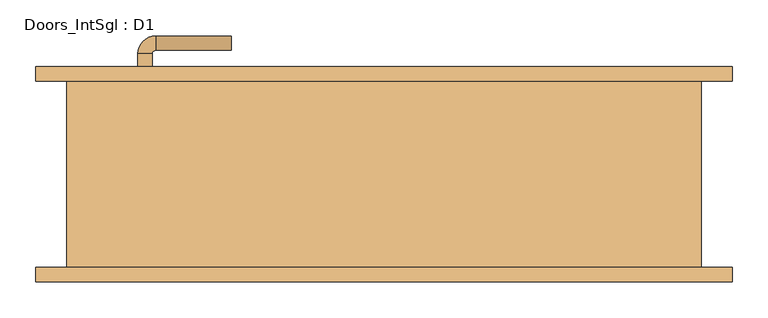
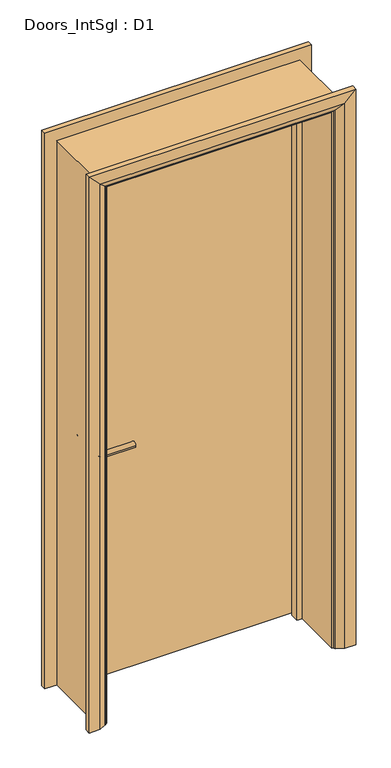
"""IFC4 building model written with IfcOpenShell, lengths in millimetres: door geometry, Doors_IntSgl : D1."""

from ifc_helpers import new_model, si_unit, point, frame, frame_2d, origin, place, context, project, spatial, polyline, circle_curve, ellipse_curve, trimmed, segment, composite_curve, outline, extrude, faceted_brep, source, transform, mapped, element, save
from ifc_brep_helpers import plane_surface, cylinder_surface, revolved_surface, advanced_brep


def doors_intsgl_d1_8eed65bb(model_context):
    return source(origin(), model_context, "Body", "SolidModel", [
        advanced_brep(
        [(-343.0, 84.0, 900.0), (-323.0, 84.0, 900.0), (-323.0, 54.0, 900.0), (-343.0, 54.0, 900.0), (-318.0, 49.0, 900.0), (-318.0, 29.0, 900.0), (-213.0, 29.0, 900.0), (-213.0, 49.0, 900.0)],
        [
            (0, 1, circle_curve(frame((-333.0, 84.0, 900.0), z_axis=(0.0, 1.0, 0.0), x_axis=(1.0, 0.0, 0.0)), 10.0)),
            (1, 0, circle_curve(frame((-333.0, 84.0, 900.0), z_axis=(0.0, 1.0, 0.0), x_axis=(1.0, 0.0, 0.0)), 10.0)),
            (1, 2),
            (2, 3, circle_curve(frame((-333.0, 54.0, 900.0), z_axis=(0.0, 1.0, 0.0), x_axis=(1.0, 0.0, 0.0)), 10.0)),
            (3, 0),
            (3, 2, circle_curve(frame((-333.0, 54.0, 900.0), z_axis=(0.0, 1.0, 0.0), x_axis=(1.0, 0.0, 0.0)), 10.0)),
            (4, 5, circle_curve(frame((-318.0, 39.0, 900.0), z_axis=(-1.0, 0.0, 0.0), x_axis=(0.0, 1.0, 0.0)), 10.0)),
            (5, 3, circle_curve(frame((-318.0, 54.0, 900.0), z_axis=(0.0, 0.0, -1.0), x_axis=(-1.0, 0.0, 0.0)), 25.0)),
            (2, 4, circle_curve(frame((-318.0, 54.0, 900.0), z_axis=(0.0, 0.0, 1.0), x_axis=(-1.0, 0.0, 0.0)), 5.0)),
            (5, 4, circle_curve(frame((-318.0, 39.0, 900.0), z_axis=(-1.0, 0.0, 0.0), x_axis=(0.0, 1.0, 0.0)), 10.0)),
            (6, 7, circle_curve(frame((-213.0, 39.0, 900.0), z_axis=(1.0, 0.0, 0.0), x_axis=(0.0, 1.0, 0.0)), 10.0)),
            (7, 6, circle_curve(frame((-213.0, 39.0, 900.0), z_axis=(1.0, 0.0, 0.0), x_axis=(0.0, 1.0, 0.0)), 10.0)),
            (4, 7),
            (6, 5),
        ],
        [
            plane_surface(frame((-333.0, 84.0, 900.0), z_axis=(0.0, 1.0, 0.0), x_axis=(0.0, 0.0, 1.0))),
            cylinder_surface(frame((-333.0, 84.0, 900.0), z_axis=(0.0, 1.0, 0.0), x_axis=(1.0, 0.0, 0.0)), 10.0),
            revolved_surface(trimmed(ellipse_curve(frame((-333.0, 54.0, 900.0), z_axis=(0.0, -1.0, 0.0), x_axis=(1.0, 0.0, 0.0)), 10.0, 10.0), [point((-343.0, 54.0, 900.0))], [point((-323.0, 54.0, 900.0))], True, "CARTESIAN"), (-318.0, 54.0, 900.0), (0.0, 0.0, -1.0)),
            revolved_surface(trimmed(ellipse_curve(frame((-333.0, 54.0, 900.0), z_axis=(0.0, -1.0, 0.0), x_axis=(1.0, 0.0, 0.0)), 10.0, 10.0), [point((-323.0, 54.0, 900.0))], [point((-343.0, 54.0, 900.0))], True, "CARTESIAN"), (-318.0, 54.0, 900.0), (0.0, 0.0, -1.0)),
            plane_surface(frame((-213.0, 39.0, 900.0), z_axis=(1.0, 0.0, 0.0), x_axis=(0.0, 0.0, 1.0))),
            cylinder_surface(frame((-318.0, 39.0, 900.0), z_axis=(-1.0, 0.0, 0.0), x_axis=(0.0, 1.0, 0.0)), 10.0),
        ],
        [
            (0, [[1, 2]]),
            (1, [[3, 4, 5, -2]]),
            (1, [[-5, 6, -3, -1]]),
            (2, [[7, 8, -4, 9]]),
            (3, [[10, -9, -6, -8]]),
            (4, [[11, 12]]),
            (5, [[13, -11, 14, -7]]),
            (5, [[-14, -12, -13, -10]]),
        ],
    ),
        extrude(outline(composite_curve([segment(trimmed(circle_curve(frame_2d((900.0, -335.5)), 30.0), [point((900.0, -365.5))], [point((900.0, -305.5))], False, "CARTESIAN"), True, "CONTINUOUS"), segment(trimmed(circle_curve(frame_2d((900.0, -335.5)), 30.0), [point((900.0, -305.5))], [point((900.0, -365.5))], False, "CARTESIAN"), True, "CONTINUOUS")], self_intersect=False)), frame((0.0, 84.0, 0.0), z_axis=(0.0, 1.0, 0.0), x_axis=(0.0, 0.0, 1.0)), (0.0, 0.0, 1.0), 8.0),
        advanced_brep(
        [(-343.0, 138.0, 900.0), (-323.0, 138.0, 900.0), (-343.0, 168.0, 900.0), (-323.0, 168.0, 900.0), (-318.0, 173.0, 900.0), (-318.0, 193.0, 900.0), (-213.0, 193.0, 900.0), (-213.0, 173.0, 900.0)],
        [
            (0, 1, circle_curve(frame((-333.0, 138.0, 900.0), z_axis=(0.0, -1.0, 0.0), x_axis=(1.0, 0.0, 0.0)), 10.0)),
            (1, 0, circle_curve(frame((-333.0, 138.0, 900.0), z_axis=(0.0, -1.0, 0.0), x_axis=(1.0, 0.0, 0.0)), 10.0)),
            (0, 2),
            (2, 3, circle_curve(frame((-333.0, 168.0, 900.0), z_axis=(0.0, -1.0, 0.0), x_axis=(1.0, 0.0, 0.0)), 10.0)),
            (3, 1),
            (3, 2, circle_curve(frame((-333.0, 168.0, 900.0), z_axis=(0.0, -1.0, 0.0), x_axis=(1.0, 0.0, 0.0)), 10.0)),
            (4, 3, circle_curve(frame((-318.0, 168.0, 900.0), z_axis=(0.0, 0.0, 1.0), x_axis=(-1.0, 0.0, 0.0)), 5.0)),
            (2, 5, circle_curve(frame((-318.0, 168.0, 900.0), z_axis=(0.0, 0.0, -1.0), x_axis=(-1.0, 0.0, 0.0)), 25.0)),
            (5, 4, circle_curve(frame((-318.0, 183.0, 900.0), z_axis=(-1.0, 0.0, 0.0), x_axis=(0.0, -1.0, 0.0)), 10.0)),
            (4, 5, circle_curve(frame((-318.0, 183.0, 900.0), z_axis=(-1.0, 0.0, 0.0), x_axis=(0.0, -1.0, 0.0)), 10.0)),
            (6, 7, circle_curve(frame((-213.0, 183.0, 900.0), z_axis=(1.0, 0.0, 0.0), x_axis=(0.0, -1.0, 0.0)), 10.0)),
            (7, 6, circle_curve(frame((-213.0, 183.0, 900.0), z_axis=(1.0, 0.0, 0.0), x_axis=(0.0, -1.0, 0.0)), 10.0)),
            (5, 6),
            (7, 4),
        ],
        [
            plane_surface(frame((-333.0, 138.0, 900.0), z_axis=(0.0, -1.0, 0.0), x_axis=(0.0, 0.0, 1.0))),
            cylinder_surface(frame((-333.0, 138.0, 900.0), z_axis=(0.0, -1.0, 0.0), x_axis=(1.0, 0.0, 0.0)), 10.0),
            revolved_surface(trimmed(ellipse_curve(frame((-333.0, 168.0, 900.0), z_axis=(0.0, -1.0, 0.0), x_axis=(1.0, 0.0, 0.0)), 10.0, 10.0), [point((-343.0, 168.0, 900.0))], [point((-323.0, 168.0, 900.0))], True, "CARTESIAN"), (-318.0, 168.0, 900.0), (0.0, 0.0, -1.0)),
            revolved_surface(trimmed(ellipse_curve(frame((-333.0, 168.0, 900.0), z_axis=(0.0, -1.0, 0.0), x_axis=(1.0, 0.0, 0.0)), 10.0, 10.0), [point((-323.0, 168.0, 900.0))], [point((-343.0, 168.0, 900.0))], True, "CARTESIAN"), (-318.0, 168.0, 900.0), (0.0, 0.0, -1.0)),
            plane_surface(frame((-213.0, 183.0, 900.0), z_axis=(1.0, 0.0, 0.0), x_axis=(0.0, 0.0, 1.0))),
            cylinder_surface(frame((-318.0, 183.0, 900.0), z_axis=(-1.0, 0.0, 0.0), x_axis=(0.0, -1.0, 0.0)), 10.0),
        ],
        [
            (0, [[1, 2]]),
            (1, [[-1, 3, 4, 5]]),
            (1, [[-2, -5, 6, -3]]),
            (2, [[7, -4, 8, 9]]),
            (3, [[-8, -6, -7, 10]]),
            (4, [[11, 12]]),
            (5, [[-9, 13, -12, 14]]),
            (5, [[-10, -14, -11, -13]]),
        ],
    ),
        extrude(outline(composite_curve([segment(trimmed(circle_curve(frame_2d((900.0, -335.5)), 30.0), [point((900.0, -365.5))], [point((900.0, -305.5))], False, "CARTESIAN"), True, "CONTINUOUS"), segment(trimmed(circle_curve(frame_2d((900.0, -335.5)), 30.0), [point((900.0, -305.5))], [point((900.0, -365.5))], False, "CARTESIAN"), True, "CONTINUOUS")], self_intersect=False)), frame((0.0, 130.0, 0.0), z_axis=(0.0, 1.0, 0.0), x_axis=(0.0, 0.0, 1.0)), (0.0, 0.0, 1.0), 8.0),
        extrude(outline(polyline([(408.0, 92.0), (-408.0, 92.0), (-408.0, 130.0), (408.0, 130.0), (408.0, 92.0)])), frame((0.0, 0.0, 8.0), z_axis=(0.0, 0.0, 1.0), x_axis=(1.0, 0.0, 0.0)), (0.0, 0.0, 1.0), 2050.0),
        advanced_brep(
        [(485.0, 150.0, 0.0), (485.0, 130.0, 0.0), (415.0, 130.0, 0.0), (419.0, 136.0, 0.0), (445.0, 150.0, 0.0), (485.0, 150.0, 2135.0), (485.0, 130.0, 2135.0), (-485.0, 130.0, 2135.0), (-485.0, 130.0, 0.0), (-415.0, 130.0, 0.0), (-415.0, 130.0, 2065.0), (415.0, 130.0, 2065.0), (419.0, 136.0, 2069.0), (445.0, 150.0, 2095.0), (-445.0, 150.0, 2095.0), (-445.0, 150.0, 0.0), (-485.0, 150.0, 0.0), (-485.0, 150.0, 2135.0), (-419.0, 136.0, 0.0), (-419.0, 136.0, 2069.0)],
        [
            (0, 1),
            (1, 2),
            (2, 3, circle_curve(frame((423.0, 129.0, 0.0), z_axis=(0.0, 0.0, -1.0), x_axis=(1.0, 0.0, 0.0)), 8.0622577)),
            (3, 4),
            (4, 0),
            (0, 5),
            (5, 6),
            (6, 1),
            (6, 7),
            (7, 8),
            (8, 9),
            (9, 10),
            (10, 11),
            (11, 2),
            (11, 12, ellipse_curve(frame((423.0, 129.0, 2073.0), z_axis=(0.7071067811865475, 0.0, -0.7071067811865475), x_axis=(-0.7071067811865474, 0.0, -0.7071067811865476)), 11.4017543, 8.0622577)),
            (12, 3),
            (12, 13),
            (13, 4),
            (13, 14),
            (14, 15),
            (15, 16),
            (16, 17),
            (17, 5),
            (7, 17),
            (16, 8),
            (15, 18),
            (18, 9, circle_curve(frame((-423.0, 129.0, 0.0), z_axis=(0.0, 0.0, -1.0), x_axis=(-1.0, 0.0, 0.0)), 8.0622577)),
            (19, 10, ellipse_curve(frame((-423.0, 129.0, 2073.0), z_axis=(-0.7071067811865475, 0.0, -0.7071067811865475), x_axis=(-0.7071067811865474, 0.0, 0.7071067811865476)), 11.4017543, 8.0622577)),
            (18, 19),
            (14, 19),
            (19, 12),
        ],
        [
            plane_surface(frame((415.0, 130.0, 0.0), z_axis=(0.0, 0.0, -1.0), x_axis=(0.0, -1.0, 0.0))),
            plane_surface(frame((485.0, 150.0, 0.0), z_axis=(1.0, 0.0, 0.0), x_axis=(0.0, 0.0, 1.0))),
            plane_surface(frame((485.0, 130.0, 0.0), z_axis=(0.0, -1.0, 0.0), x_axis=(0.0, 0.0, 1.0))),
            cylinder_surface(frame((423.0, 129.0, 0.0), z_axis=(0.0, 0.0, -1.0), x_axis=(1.0, 0.0, 0.0)), 8.0622577),
            plane_surface(frame((419.0, 136.0, 0.0), z_axis=(-0.4740998230350126, 0.880471099922178, 0.0), x_axis=(0.0, 0.0, 1.0))),
            plane_surface(frame((445.0, 150.0, 0.0), z_axis=(0.0, 1.0, 0.0), x_axis=(0.0, 0.0, 1.0))),
            plane_surface(frame((-485.0, 150.0, 2135.0), z_axis=(-1.0, 0.0, 0.0), x_axis=(0.0, 0.0, -1.0))),
            plane_surface(frame((-415.0, 130.0, 0.0), z_axis=(0.0, 0.0, -1.0), x_axis=(0.0, -1.0, 0.0))),
            cylinder_surface(frame((-423.0, 129.0, 2065.0), z_axis=(0.0, 0.0, 1.0), x_axis=(-1.0, 0.0, 0.0)), 8.0622577),
            plane_surface(frame((-419.0, 136.0, 2069.0), z_axis=(0.47409982303501824, 0.8804710999221749, 0.0), x_axis=(0.0, 0.0, -1.0))),
            plane_surface(frame((485.0, 150.0, 2135.0), z_axis=(0.0, 0.0, 1.0), x_axis=(-1.0, 0.0, 0.0))),
            cylinder_surface(frame((415.0, 129.0, 2073.0), z_axis=(1.0, 0.0, 0.0), x_axis=(0.0, 0.0, 1.0)), 8.0622577),
            plane_surface(frame((419.0, 136.0, 2069.0), z_axis=(0.0, 0.8804710999221764, -0.4740998230350154), x_axis=(-1.0, 0.0, 0.0))),
        ],
        [
            (0, [[1, 2, 3, 4, 5]]),
            (1, [[-1, 6, 7, 8]]),
            (2, [[-2, -8, 9, 10, 11, 12, 13, 14]]),
            (3, [[-3, -14, 15, 16]]),
            (4, [[-4, -16, 17, 18]]),
            (5, [[-5, -18, 19, 20, 21, 22, 23, -6]]),
            (6, [[24, -22, 25, -10]]),
            (7, [[-21, 26, 27, -11, -25]]),
            (8, [[28, -12, -27, 29]]),
            (9, [[30, -29, -26, -20]]),
            (10, [[-7, -23, -24, -9]]),
            (11, [[-15, -13, -28, 31]]),
            (12, [[-17, -31, -30, -19]]),
        ],
    ),
        extrude(outline(polyline([(0.0, -410.0), (0.0, -391.0), (2041.0, -391.0), (2041.0, 391.0), (0.0, 391.0), (0.0, 410.0), (2060.0, 410.0), (2060.0, -410.0), (0.0, -410.0)])), frame((0.0, 58.0, 0.0), z_axis=(0.0, 1.0, 0.0), x_axis=(0.0, 0.0, 1.0)), (0.0, 0.0, 1.0), 32.0),
        advanced_brep(
        [(-485.0, -150.0, 0.0), (-485.0, -130.0, 0.0), (-415.0, -130.0, 0.0), (-419.0, -136.0, 0.0), (-445.0, -150.0, 0.0), (-485.0, -150.0, 2135.0), (-485.0, -130.0, 2135.0), (-415.0, -130.0, 2065.0), (-419.0, -136.0, 2069.0), (-445.0, -150.0, 2095.0), (485.0, -150.0, 0.0), (445.0, -150.0, 0.0), (419.0, -136.0, 0.0), (415.0, -130.0, 0.0), (485.0, -130.0, 0.0), (485.0, -150.0, 2135.0), (445.0, -150.0, 2095.0), (419.0, -136.0, 2069.0), (415.0, -130.0, 2065.0), (485.0, -130.0, 2135.0)],
        [
            (0, 1),
            (1, 2),
            (2, 3, circle_curve(frame((-423.0, -129.0, 0.0), z_axis=(0.0, 0.0, -1.0), x_axis=(-1.0, 0.0, 0.0)), 8.0622577)),
            (3, 4),
            (4, 0),
            (0, 5),
            (5, 6),
            (6, 1),
            (6, 7),
            (7, 2),
            (7, 8, ellipse_curve(frame((-423.0, -129.0, 2073.0), z_axis=(-0.7071067811865475, 0.0, -0.7071067811865475), x_axis=(0.7071067811865474, 0.0, -0.7071067811865476)), 11.4017543, 8.0622577)),
            (8, 3),
            (8, 9),
            (9, 4),
            (9, 5),
            (10, 11),
            (11, 12),
            (12, 13, circle_curve(frame((423.0, -129.0, 0.0), z_axis=(0.0, 0.0, -1.0), x_axis=(1.0, 0.0, 0.0)), 8.0622577)),
            (13, 14),
            (14, 10),
            (15, 16),
            (16, 11),
            (10, 15),
            (16, 17),
            (17, 12),
            (17, 18, ellipse_curve(frame((423.0, -129.0, 2073.0), z_axis=(0.7071067811865475, 0.0, -0.7071067811865475), x_axis=(0.7071067811865474, 0.0, 0.7071067811865476)), 11.4017543, 8.0622577)),
            (18, 13),
            (18, 19),
            (19, 14),
            (19, 15),
            (5, 15),
            (19, 6),
            (18, 7),
            (17, 8),
            (16, 9),
        ],
        [
            plane_surface(frame((-415.0, -202.8010989, 0.0), z_axis=(0.0, 0.0, -1.0), x_axis=(1.0, 0.0, 0.0))),
            plane_surface(frame((-485.0, -150.0, 0.0), z_axis=(-1.0, 0.0, 0.0), x_axis=(0.0, 0.0, 1.0))),
            plane_surface(frame((-485.0, -130.0, 0.0), z_axis=(0.0, 1.0, 0.0), x_axis=(0.0, 0.0, 1.0))),
            cylinder_surface(frame((-423.0, -129.0, 0.0), z_axis=(0.0, 0.0, -1.0), x_axis=(-1.0, 0.0, 0.0)), 8.0622577),
            plane_surface(frame((-419.0, -136.0, 0.0), z_axis=(0.4740998230350183, -0.8804710999221749, 0.0), x_axis=(0.0, 0.0, 1.0))),
            plane_surface(frame((-445.0, -150.0, 0.0), z_axis=(0.0, -1.0, 0.0), x_axis=(0.0, 0.0, 1.0))),
            plane_surface(frame((415.0, -202.8010989, 0.0), z_axis=(0.0, 0.0, -1.0), x_axis=(-1.0, 0.0, 0.0))),
            plane_surface(frame((445.0, -150.0, 2095.0), z_axis=(0.0, -1.0, 0.0), x_axis=(0.0, 0.0, -1.0))),
            plane_surface(frame((419.0, -136.0, 2069.0), z_axis=(-0.4740998230350183, -0.8804710999221749, 0.0), x_axis=(0.0, 0.0, -1.0))),
            cylinder_surface(frame((423.0, -129.0, 2065.0), z_axis=(0.0, 0.0, 1.0), x_axis=(1.0, 0.0, 0.0)), 8.0622577),
            plane_surface(frame((485.0, -130.0, 2135.0), z_axis=(0.0, 1.0, 0.0), x_axis=(0.0, 0.0, -1.0))),
            plane_surface(frame((485.0, -150.0, 2135.0), z_axis=(1.0, 0.0, 0.0), x_axis=(0.0, 0.0, -1.0))),
            plane_surface(frame((-485.0, -150.0, 2135.0), z_axis=(0.0, 0.0, 1.0), x_axis=(1.0, 0.0, 0.0))),
            plane_surface(frame((-485.0, -130.0, 2135.0), z_axis=(0.0, 1.0, 0.0), x_axis=(1.0, 0.0, 0.0))),
            cylinder_surface(frame((-415.0, -129.0, 2073.0), z_axis=(-1.0, 0.0, 0.0), x_axis=(0.0, 0.0, 1.0)), 8.0622577),
            plane_surface(frame((-419.0, -136.0, 2069.0), z_axis=(0.0, -0.8804710999221749, -0.4740998230350183), x_axis=(1.0, 0.0, 0.0))),
            plane_surface(frame((-445.0, -150.0, 2095.0), z_axis=(0.0, -1.0, 0.0), x_axis=(1.0, 0.0, 0.0))),
        ],
        [
            (0, [[1, 2, 3, 4, 5]]),
            (1, [[-1, 6, 7, 8]]),
            (2, [[-2, -8, 9, 10]]),
            (3, [[-3, -10, 11, 12]]),
            (4, [[-4, -12, 13, 14]]),
            (5, [[-5, -14, 15, -6]]),
            (6, [[16, 17, 18, 19, 20]]),
            (7, [[21, 22, -16, 23]]),
            (8, [[24, 25, -17, -22]]),
            (9, [[26, 27, -18, -25]]),
            (10, [[28, 29, -19, -27]]),
            (11, [[30, -23, -20, -29]]),
            (12, [[-7, 31, -30, 32]]),
            (13, [[-9, -32, -28, 33]]),
            (14, [[-11, -33, -26, 34]]),
            (15, [[-13, -34, -24, 35]]),
            (16, [[-15, -35, -21, -31]]),
        ],
    ),
        faceted_brep([(-410.0, 130.0, 0.0), (-410.0, -130.0, 0.0), (-442.0, -130.0, 0.0), (-442.0, 130.0, 0.0), (-410.0, 130.0, 2060.0), (-410.0, -130.0, 2060.0), (-442.0, -130.0, 2092.0), (-442.0, 130.0, 2092.0), (410.0, 130.0, 0.0), (442.0, 130.0, 0.0), (442.0, -130.0, 0.0), (410.0, -130.0, 0.0), (410.0, 130.0, 2060.0), (442.0, 130.0, 2092.0), (442.0, -130.0, 2092.0), (410.0, -130.0, 2060.0)], [[[0, 1, 2, 3]], [[1, 0, 4, 5]], [[2, 1, 5, 6]], [[3, 2, 6, 7]], [[0, 3, 7, 4]], [[8, 9, 10, 11]], [[12, 13, 9, 8]], [[13, 14, 10, 9]], [[14, 15, 11, 10]], [[15, 12, 8, 11]], [[5, 4, 12, 15]], [[6, 5, 15, 14]], [[7, 6, 14, 13]], [[4, 7, 13, 12]]]),
    ])


if __name__ == "__main__":
    model = new_model("IFC4")
    model_context = context("Model", 3, world=origin())
    ifc_project = project(units=[si_unit("LENGTHUNIT", "METRE", prefix="MILLI")], contexts=[model_context])
    site = spatial("IfcSite", under=ifc_project)
    building = spatial("IfcBuilding", under=site)
    placement = place(None, origin())
    doors_intsgl_d1_shape = doors_intsgl_d1_8eed65bb(model_context)
    element("IfcDoor", 1, ObjectType="Doors_IntSgl : D1", at=placement, inside=building, context=model_context, shape_type="MappedRepresentation", body=[
        mapped(doors_intsgl_d1_shape, transform((0.0, 0.0, 0.0), x_axis=(1.0, 0.0, 0.0), y_axis=(0.0, 1.0, 0.0), z_axis=(0.0, 0.0, 1.0))),
    ])
    save(model, "model.ifc")

# Revit data of these elements
# Type "Doors_IntSgl : D1"
#   Type Mark = "46"
#   Type Comments = "Internal Single"
#   Operation = "SingleSwingRight"
#   Manufacturer = "Revit"
#   Keynote = "L20"
#   Description = "Internal Single Door"
#   Analytic Construction = "Metal"
#   UnderCut = 8 mm
#   Tolerance = 2 mm
#   Thickness = 38 mm
#   Thermal Resistance (R) = 0.270117 (m²·K)/W
#   Structural Tolerance = 8 mm
#   StopDepth = 32 mm
#   Stop Thickness = 19 mm
#   Rough Width = 900 mm
#   Rough Height = 2100 mm
#   Height to Top Lock Rail = 1000 mm
#   Heat Transfer Coefficient (U) = 3.7021 W/(m²·K)
#   Handle Z Distance = 900 mm
#   Handle X Distance = 75 mm
#   Frame Thickness = 32 mm
#   Door Panel Width = 816 mm
#   Door Panel Thickness = 38 mm
#   Door Panel Offset = 0 mm
#   Height = 2100 mm
#   Width = 900 mm
#   Door Panel Height = 2050 mm
#   Architrave Setback = 5 mm
#   Vis - Ironmongery = yes
#   Material Ironmongery = Door - Handle
#   Material Frame = Door - Frame/Mullion (1)
#   Material Door = Door - Panel
#   Material Architrave = Door - Architrave
#   Visual Light Transmittance = 0
#   Solar Heat Gain Coefficient = 0
#   Function = (empty or 0)
#   Wall Closure = (empty or 0)
# Element 1 (IfcDoor, "Doors_IntSgl : D1")
#   Materials on its faces: "Door - Architrave", "Door - Handle", "Door - Frame/Mullion (1)", "Door - Panel"
# Materials
#   "Door - Handle": colour RGB 0 0 0, transparency 0, Keynote = "P21", Cost = 0
#   "Door - Frame/Mullion (1)": class "Wood", colour RGB 212 179 113, transparency 0, Keynote = "L20", Cost = 0
#   "Door - Panel": class "Wood", colour RGB 210 159 95, transparency 0, Keynote = "L20", Cost = 0
#   "Door - Architrave": class "Wood", colour RGB 154 90 5, transparency 0, Keynote = "P20", Cost = 0
